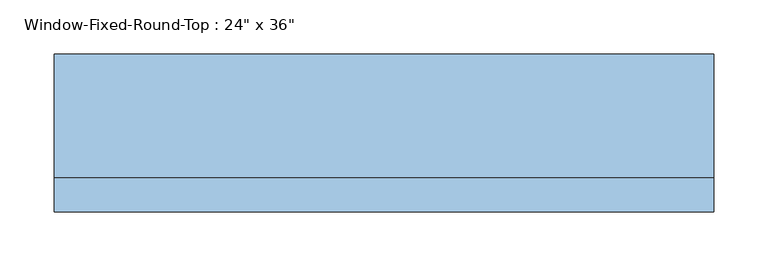
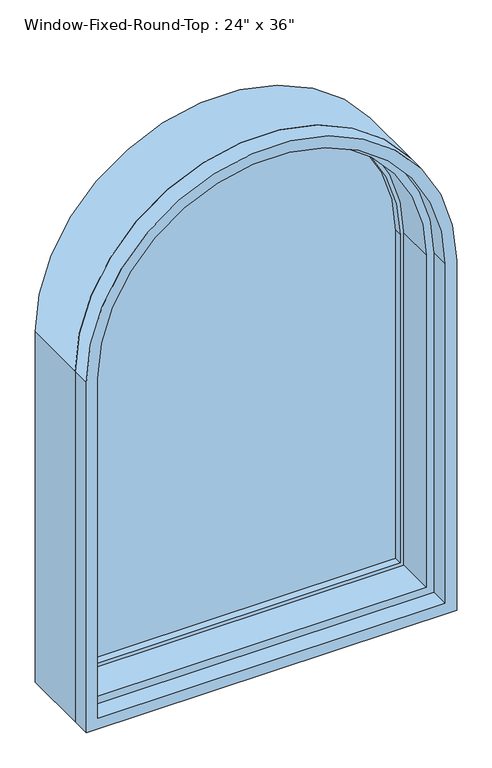
"""IFC4 building model written with IfcOpenShell, lengths in millimetres: window geometry."""

from ifc_helpers import new_model, si_unit, point, frame, frame_2d, origin, place, context, project, spatial, polyline, circle_curve, trimmed, segment, composite_curve, outline, extrude, source, transform, mapped, element, save
from ifc_brep_helpers import plane_surface, cylinder_surface, revolved_surface, advanced_brep


def window_d6aed77d(model_context):
    return source(origin(), model_context, "Body", "SolidModel", [
        advanced_brep(
        [(-273.05, 31.75, 1524.0), (-273.05, -31.75, 1524.0), (-273.05, -31.75, 946.15), (-273.05, 31.75, 946.15), (-292.1, 82.55, 1524.0), (-292.1, 31.75, 1524.0), (-292.1, 31.75, 927.1), (-292.1, 82.55, 927.1), (-304.8, -31.75, 1524.0), (-304.8, 82.55, 1524.0), (-304.8, 82.55, 914.4), (-304.8, -31.75, 914.4), (273.05, -31.75, 946.15), (273.05, 31.75, 946.15), (292.1, 31.75, 927.1), (292.1, 82.55, 927.1), (304.8, 82.55, 914.4), (304.8, -31.75, 914.4), (273.05, -31.75, 1524.0), (273.05, 31.75, 1524.0), (292.1, 31.75, 1524.0), (292.1, 82.55, 1524.0), (304.8, 82.55, 1524.0), (304.8, -31.75, 1524.0)],
        [
            (0, 1),
            (1, 2),
            (2, 3),
            (3, 0),
            (4, 5),
            (5, 6),
            (6, 7),
            (7, 4),
            (8, 9),
            (9, 10),
            (10, 11),
            (11, 8),
            (2, 12),
            (12, 13),
            (13, 3),
            (6, 14),
            (14, 15),
            (15, 7),
            (10, 16),
            (16, 17),
            (17, 11),
            (12, 18),
            (18, 19),
            (19, 13),
            (14, 20),
            (20, 21),
            (21, 15),
            (16, 22),
            (22, 23),
            (23, 17),
            (23, 8, circle_curve(frame((0.0, -31.75, 1524.0), z_axis=(0.0, -1.0, 0.0), x_axis=(1.0, 0.0, 0.0)), 304.8)),
            (1, 18, circle_curve(frame((0.0, -31.75, 1524.0), z_axis=(0.0, 1.0, 0.0), x_axis=(1.0, 0.0, 0.0)), 273.05)),
            (0, 19, circle_curve(frame((0.0, 31.75, 1524.0), z_axis=(0.0, 1.0, 0.0), x_axis=(1.0, 0.0, 0.0)), 273.05)),
            (5, 20, circle_curve(frame((0.0, 31.75, 1524.0), z_axis=(0.0, 1.0, 0.0), x_axis=(1.0, 0.0, 0.0)), 292.1)),
            (4, 21, circle_curve(frame((0.0, 82.55, 1524.0), z_axis=(0.0, 1.0, 0.0), x_axis=(1.0, 0.0, 0.0)), 292.1)),
            (9, 22, circle_curve(frame((0.0, 82.55, 1524.0), z_axis=(0.0, 1.0, 0.0), x_axis=(1.0, 0.0, 0.0)), 304.8)),
        ],
        [
            plane_surface(frame((-273.05, -31.75, 1524.0), z_axis=(1.0, 0.0, 0.0), x_axis=(0.0, 0.0, -1.0))),
            plane_surface(frame((-292.1, 31.75, 1524.0), z_axis=(1.0, 0.0, 0.0), x_axis=(0.0, 0.0, -1.0))),
            plane_surface(frame((-304.8, 82.55, 1524.0), z_axis=(-1.0, 0.0, 0.0), x_axis=(0.0, 0.0, -1.0))),
            plane_surface(frame((-273.05, -31.75, 946.15), z_axis=(0.0, 0.0, 1.0), x_axis=(1.0, 0.0, 0.0))),
            plane_surface(frame((-292.1, 31.75, 927.1), z_axis=(0.0, 0.0, 1.0), x_axis=(1.0, 0.0, 0.0))),
            plane_surface(frame((-304.8, 82.55, 914.4), z_axis=(0.0, 0.0, -1.0), x_axis=(1.0, 0.0, 0.0))),
            plane_surface(frame((273.05, -31.75, 946.15), z_axis=(-1.0, 0.0, 0.0), x_axis=(0.0, 0.0, 1.0))),
            plane_surface(frame((292.1, 31.75, 927.1), z_axis=(-1.0, 0.0, 0.0), x_axis=(0.0, 0.0, 1.0))),
            plane_surface(frame((304.8, 82.55, 914.4), z_axis=(1.0, 0.0, 0.0), x_axis=(0.0, 0.0, 1.0))),
            plane_surface(frame((0.0, -31.75, 1524.0), z_axis=(0.0, -1.0, 0.0), x_axis=(1.0, 0.0, 0.0))),
            revolved_surface(polyline([(273.05, -31.75, 1524.0), (273.05, 31.75, 1524.0)]), (0.0, 76.2, 1524.0), (0.0, -1.0, 0.0)),
            plane_surface(frame((0.0, 31.75, 1524.0), z_axis=(0.0, 1.0, 0.0), x_axis=(1.0, 0.0, 0.0))),
            revolved_surface(polyline([(292.1, 31.75, 1524.0), (292.1, 82.55, 1524.0)]), (0.0, 76.2, 1524.0), (0.0, -1.0, 0.0)),
            plane_surface(frame((0.0, 82.55, 1524.0), z_axis=(0.0, 1.0, 0.0), x_axis=(1.0, 0.0, 0.0))),
            cylinder_surface(frame((0.0, 76.2, 1524.0), z_axis=(0.0, -1.0, 0.0), x_axis=(1.0, 0.0, 0.0)), 304.8),
        ],
        [
            (0, [[1, 2, 3, 4]]),
            (1, [[5, 6, 7, 8]]),
            (2, [[9, 10, 11, 12]]),
            (3, [[-3, 13, 14, 15]]),
            (4, [[-7, 16, 17, 18]]),
            (5, [[-11, 19, 20, 21]]),
            (6, [[-14, 22, 23, 24]]),
            (7, [[-17, 25, 26, 27]]),
            (8, [[-20, 28, 29, 30]]),
            (9, [[-21, -30, 31, -12], [32, -22, -13, -2]]),
            (10, [[33, -23, -32, -1]]),
            (11, [[34, -25, -16, -6], [-15, -24, -33, -4]]),
            (12, [[35, -26, -34, -5]]),
            (13, [[36, -28, -19, -10], [-18, -27, -35, -8]]),
            (14, [[-31, -29, -36, -9]]),
        ],
    ),
        extrude(outline(composite_curve([segment(trimmed(circle_curve(frame_2d((1524.0, 0.0)), 304.8), [point((1524.0, 304.8))], [point((1524.0, -304.8))], False, "CARTESIAN"), True, "CONTINUOUS"), segment(polyline([(1524.0, -304.8), (914.4, -304.8), (914.4, 304.8), (1524.0, 304.8)]), True, "CONTINUOUS")], self_intersect=False), holes=[composite_curve([segment(polyline([(1524.0, 285.75), (933.45, 285.75), (933.45, -285.75), (1524.0, -285.75)]), True, "CONTINUOUS"), segment(trimmed(circle_curve(frame_2d((1524.0, 0.0)), 285.75), [point((1524.0, -285.75))], [point((1524.0, 285.75))], True, "CARTESIAN"), True, "CONTINUOUS")], self_intersect=False)]), frame((0.0, -63.5, 0.0), z_axis=(0.0, 1.0, 0.0), x_axis=(0.0, 0.0, 1.0)), (0.0, 0.0, 1.0), 31.75),
        extrude(outline(composite_curve([segment(polyline([(927.1, 292.1), (1524.0, 292.1)]), True, "CONTINUOUS"), segment(trimmed(circle_curve(frame_2d((1524.0, 0.0)), 292.1), [point((1524.0, 292.1))], [point((1524.0, -292.1))], False, "CARTESIAN"), True, "CONTINUOUS"), segment(polyline([(1524.0, -292.1), (927.1, -292.1), (927.1, 292.1)]), True, "CONTINUOUS")], self_intersect=False), holes=[composite_curve([segment(polyline([(952.5, -266.7), (1524.0, -266.7)]), True, "CONTINUOUS"), segment(trimmed(circle_curve(frame_2d((1524.0, 0.0)), 266.7), [point((1524.0, -266.7))], [point((1524.0, 266.7))], True, "CARTESIAN"), True, "CONTINUOUS"), segment(polyline([(1524.0, 266.7), (952.5, 266.7), (952.5, -266.7)]), True, "CONTINUOUS")], self_intersect=False)]), frame((0.0, 31.75, 0.0), z_axis=(0.0, 1.0, 0.0), x_axis=(0.0, 0.0, 1.0)), (0.0, 0.0, 1.0), 31.75),
        extrude(outline(composite_curve([segment(trimmed(circle_curve(frame_2d((1524.0, 0.0)), 266.7), [point((1524.0, 266.7))], [point((1524.0, -266.7))], False, "CARTESIAN"), True, "CONTINUOUS"), segment(polyline([(1524.0, -266.7), (952.5, -266.7), (952.5, 266.7), (1524.0, 266.7)]), True, "CONTINUOUS")], self_intersect=False)), frame((0.0, 57.15, 0.0), z_axis=(0.0, 1.0, 0.0), x_axis=(0.0, 0.0, 1.0)), (0.0, 0.0, 1.0), 6.35),
        extrude(outline(composite_curve([segment(trimmed(circle_curve(frame_2d((1524.0, 0.0)), 266.7), [point((1524.0, 266.7))], [point((1524.0, -266.7))], False, "CARTESIAN"), True, "CONTINUOUS"), segment(polyline([(1524.0, -266.7), (952.5, -266.7), (952.5, 266.7), (1524.0, 266.7)]), True, "CONTINUOUS")], self_intersect=False)), frame((0.0, 44.45, 0.0), z_axis=(0.0, 1.0, 0.0), x_axis=(0.0, 0.0, 1.0)), (0.0, 0.0, 1.0), 6.35),
        extrude(outline(composite_curve([segment(polyline([(1524.0, -292.1), (927.1, -292.1), (927.1, 292.1), (1524.0, 292.1)]), True, "CONTINUOUS"), segment(trimmed(circle_curve(frame_2d((1524.0, 0.0)), 292.1), [point((1524.0, 292.1))], [point((1524.0, -292.1))], False, "CARTESIAN"), True, "CONTINUOUS")], self_intersect=False), holes=[composite_curve([segment(polyline([(1524.0, 266.7), (952.5, 266.7), (952.5, -266.7), (1524.0, -266.7)]), True, "CONTINUOUS"), segment(trimmed(circle_curve(frame_2d((1524.0, 0.0)), 266.7), [point((1524.0, -266.7))], [point((1524.0, 266.7))], True, "CARTESIAN"), True, "CONTINUOUS")], self_intersect=False)]), frame((0.0, 63.5, 0.0), z_axis=(0.0, 1.0, 0.0), x_axis=(0.0, 0.0, 1.0)), (0.0, 0.0, 1.0), 12.7),
    ])


if __name__ == "__main__":
    model = new_model("IFC4")
    model_context = context("Model", 3, world=origin())
    ifc_project = project(units=[si_unit("LENGTHUNIT", "METRE", prefix="MILLI")], contexts=[model_context])
    site = spatial("IfcSite", under=ifc_project)
    building = spatial("IfcBuilding", under=site)
    placement = place(None, origin())
    window_shape = window_d6aed77d(model_context)
    element("IfcWindow", 1, ObjectType="Window-Fixed-Round-Top : 24\" x 36\"", at=placement, inside=building, context=model_context, shape_type="MappedRepresentation", body=[
        mapped(window_shape, transform((0.0, 0.0, 0.0), x_axis=(1.0, 0.0, 0.0), y_axis=(0.0, 1.0, 0.0), z_axis=(0.0, 0.0, 1.0))),
    ])
    save(model, "model.ifc")

# Revit data of these elements
# Type "Window-Fixed-Round-Top : 24\" x 36\""
#   Type Mark = "31"
#   Fire Rating = "0.5h"
#   Assembly Code = "B2020100"
#   Analytic Construction = "Double glazing - domestic"
#   Window Inset [instance default] = 0' - 0"
#   Wall Thickness [instance default] = 0' - 6"
#   Visual Light Transmittance = 0.81
#   Thermal Resistance (R) = 1.8146 (h·ft²·°F)/BTU
#   Solar Heat Gain Coefficient = 0.76
#   Rough Width = 2' - 0 1/2"
#   Rough Height = 3' - 0 1/2"
#   Interior Wall Closure [instance default] = 0' - 2 1/4"
#   Height = 3' - 0"
#   Heat Transfer Coefficient (U) = 0.5511 BTU/(h·ft²·°F)
#   Frame Extension [instance default] = 0' - 0 1/4"
#   Exterior Wall Closure [instance default] = 0' - 1 1/4"
#   Extension Jamb [instance default] = 0' - 2 1/4"
#   Default Sill Height = 3' - 0"
#   Width = 2' - 0"
#   Interior Trim Visibility [instance default] = yes
#   Exterior Trim Visibility [instance default] = yes
#   Extension Jamb Visibility [instance default] = yes
#   Interior Trim Material = Wood - Stained
#   Interior Trim = Trim-Window-Interior-Flat-Arch-Top-Tree_Centered : Picture Frame
#   Interior Frame Material = Wood - Stained
#   Glass Panel Material = Glass
#   Exterior Trim Material = Clad - White
#   Exterior Trim = Trim-Window-Exterior-Flat-Arch-Top-Tree_Centered : with Sill
#   Exterior Frame Material = Clad - White
#   Wall Closure = (empty or 0)
# Element 1 (IfcWindow, "Window-Fixed-Round-Top : 24\" x 36\"")
#   Wall Thickness = 0' - 5"
#   Extension Jamb = 0' - 1 1/4"
#   Materials on its faces: "Wood - Stained", "Clad - White", "Glass"
# Materials
#   "Wood - Stained": class "Wood", colour RGB 224 178 126, transparency 0, Cost = 0
#   "Glass": class "Glass", colour RGB 0 128 192, transparency 0.75, Description = "Soda Lime Glass", Cost = 0
#   "Clad - White": class "Wood", colour RGB 242 242 238, transparency 0, Cost = 0
